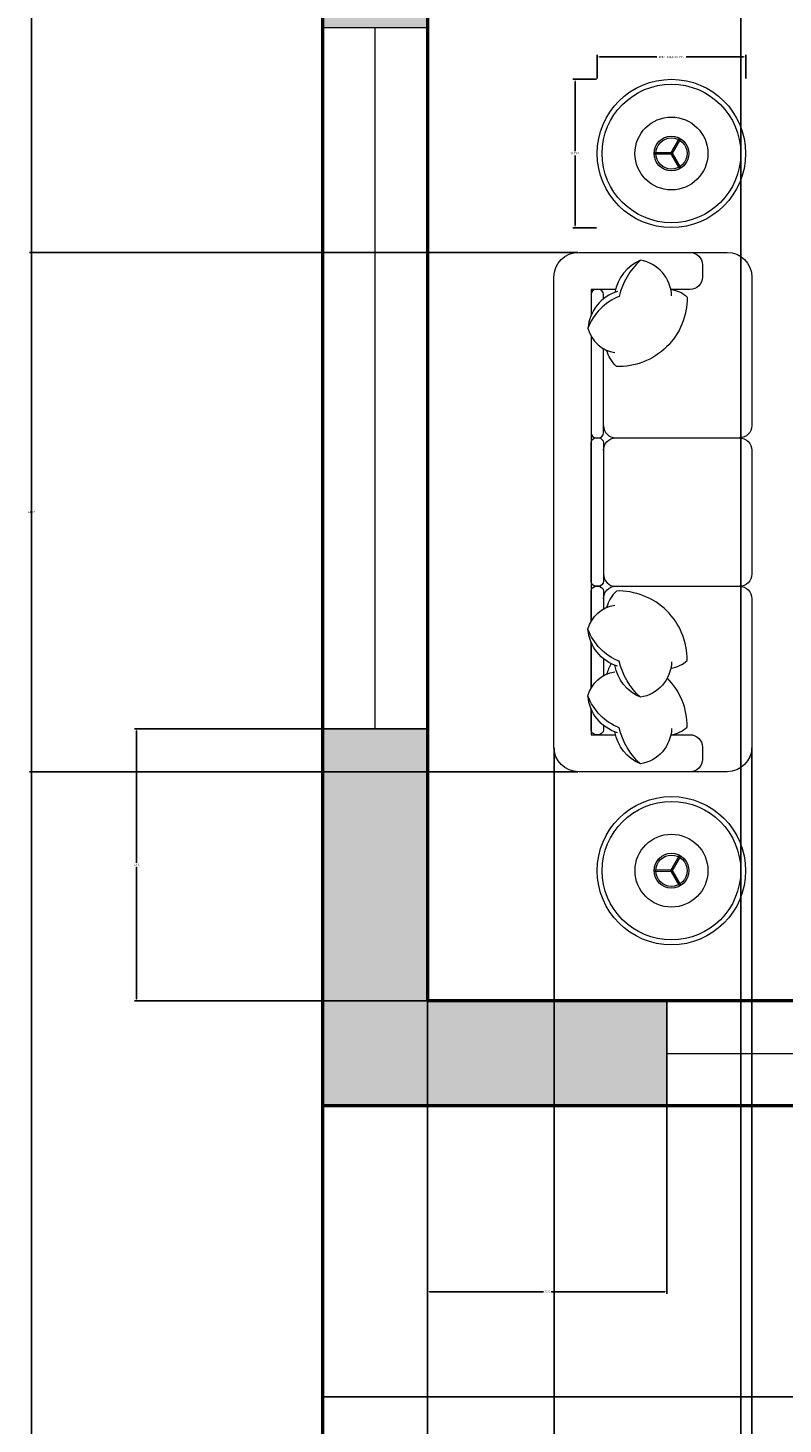
# Model space of a CAD drawing. Units: inches. Extents: x 3 to 380, y -485 to 60.
# Tile 2 of 8: x 3 to 67, y -390 to -270. Entities that reach past the tile are written whole.
import ezdxf

# ---------------------------------------------------------------- set-up
doc = ezdxf.new("R2010")
doc.units = ezdxf.units.IN
doc.header["$MEASUREMENT"] = 0
for name, color, linetype, lineweight in [('A-ANNO-DIMS', 2, 'Continuous', 18), ('A-FURN', 8, 'Continuous', 18), ('A-GLAZ', 4, 'Continuous', 18), ('A-WALL', 7, 'Continuous', 50), ('A-WALL-PATT', 252, 'Continuous', 13)]:
    doc.layers.add(name, color=color, linetype=linetype, lineweight=lineweight)
doc.styles.get("Standard").update_dxf_attribs({"font": 'arial.ttf'})
doc.dimstyles.get("Standard").update_dxf_attribs({"dimtxt": 0.18, "dimasz": 0.18, "dimexe": 0.18, "dimexo": 0.0625, "dimgap": 0.09, "dimtad": 0, "dimtih": 1, "dimtoh": 1, "dimdec": 0, "dimzin": 0, "dimdsep": 46, "dimlunit": 3, "dimtxsty": 'Standard', "dimcen": 0.09, "dimadec": 0, "dimazin": 0, "dimtfac": 1, "dimtdec": 0, "dimtofl": 0, "dimtmove": 0, "dimatfit": 3, "dimfxl": 1, "dimtolj": 1, "dimtzin": 0, "dimarcsym": 0})

# ---------------------------------------------------------------- blocks, each defined once
blk = doc.blocks.new('LIVING-END-TABLE')
at = {"ltscale": 0.03}
for p, q in [((6.3, 6.39), (7.04, 7.68)), ((6.41, 6.32), (7.16, 7.61)), ((6.35, 6.42), (4.86, 6.42)), ((6.35, 6.29), (4.86, 6.29)), ((6.3, 6.32), (7.04, 5.03)), ((6.41, 6.39), (7.16, 5.09))]:
    blk.add_line(p, q, dxfattribs=at)
for radius in [6.35, 3.12, 1.49, 1.34]:
    blk.add_circle((6.35, 6.35), radius, dxfattribs=at)
blk.add_circle((6.35, 6.35), 5.93)
blk = doc.blocks.new('WIN-60X9')
for p, q in [((60, 9), (0, 9)), ((0, 9), (0, 0)), ((60, 0), (60, 9)), ((0, 4.5), (60, 4.5)), ((0, 0), (60, 0))]:
    blk.add_line(p, q)
blk = doc.blocks.new('WIN-60X9-SPLIT-JAMB')
for p, q in [((60, 9), (0, 9)), ((0, 9), (0, 0)), ((60, 4.5), (60, 9)), ((0, 4.5), (60, 4.5)), ((60, 4.5), (60, 0)), ((0, 0), (60, 0))]:
    blk.add_line(p, q)
blk = doc.blocks.new('*D37')
at = {"layer": 'A-ANNO-DIMS', "color": 0, "lineweight": -2, "transparency": 16777216}
for p, q in [((51.37, -274.46), (51.37, -272.43)), ((64.08, -274.46), (64.08, -272.43)), ((51.55, -272.61), (56.47, -272.61)), ((63.9, -272.61), (58.98, -272.61))]:
    blk.add_line(p, q, dxfattribs=at)
at = {"layer": 'A-ANNO-DIMS', "color": 0, "transparency": 16777216}
for points in [[(51.55, -272.58), (51.55, -272.64), (51.37, -272.61)], [(63.9, -272.58), (63.9, -272.64), (64.08, -272.61)]]:
    blk.add_solid(points, dxfattribs=at)
at = {"layer": 'Defpoints', "color": 0, "transparency": 16777216}
for p in [(64.08, -272.61), (51.37, -274.52), (64.08, -274.52)]:
    blk.add_point(p, dxfattribs=at)
at = {"layer": 'A-ANNO-DIMS', "color": 0, "transparency": 16777216, "insert": (57.72, -272.61), "char_height": 0.18, "attachment_point": 5}
blk.add_mtext('\\A1;END TABLE 13 TYP.', dxfattribs=at)
blk = doc.blocks.new('*D38')
at = {"layer": 'A-ANNO-DIMS', "color": 0, "lineweight": -2, "transparency": 16777216}
for p, q in [((51.31, -274.52), (49.29, -274.52)), ((49.47, -274.7), (49.47, -280.69)), ((49.47, -287.05), (49.47, -281.06)), ((51.31, -287.23), (49.29, -287.23))]:
    blk.add_line(p, q, dxfattribs=at)
at = {"layer": 'A-ANNO-DIMS', "color": 0, "transparency": 16777216}
for points in [[(49.44, -274.7), (49.5, -274.7), (49.47, -274.52)], [(49.44, -287.05), (49.5, -287.05), (49.47, -287.23)]]:
    blk.add_solid(points, dxfattribs=at)
at = {"layer": 'Defpoints', "color": 0, "transparency": 16777216}
for p in [(49.47, -274.52), (51.37, -274.52), (51.37, -287.23)]:
    blk.add_point(p, dxfattribs=at)
at = {"layer": 'A-ANNO-DIMS', "color": 0, "transparency": 16777216, "insert": (49.47, -280.87), "char_height": 0.18, "attachment_point": 5}
blk.add_mtext('\\A1;13 TYP.', dxfattribs=at)
blk = doc.blocks.new('*D50')
at = {"layer": 'A-ANNO-DIMS', "color": 0, "lineweight": -2, "transparency": 16777216}
for p, q in [((27.78, 15.16), (2.76, 15.16)), ((2.94, 14.98), (2.94, -222.4)), ((2.94, -460.16), (2.94, -222.77)), ((27.78, -460.34), (2.76, -460.34))]:
    blk.add_line(p, q, dxfattribs=at)
at = {"layer": 'A-ANNO-DIMS', "color": 0, "transparency": 16777216}
for points in [[(2.91, 14.98), (2.97, 14.98), (2.94, 15.16)], [(2.91, -460.16), (2.97, -460.16), (2.94, -460.34)]]:
    blk.add_solid(points, dxfattribs=at)
at = {"layer": 'Defpoints', "color": 0, "transparency": 16777216}
for p in [(2.94, 15.16), (27.84, 15.16), (27.84, -460.34)]:
    blk.add_point(p, dxfattribs=at)
at = {"layer": 'A-ANNO-DIMS', "color": 0, "transparency": 16777216, "insert": (2.94, -222.59), "char_height": 0.18, "attachment_point": 5}
blk.add_mtext('\\A1;475.5', dxfattribs=at)
blk = doc.blocks.new('*D52')
at = {"layer": 'A-ANNO-DIMS', "color": 0, "lineweight": -2, "transparency": 16777216}
for p, q in [((27.84, -362.49), (27.84, -387.51)), ((168.84, -362.49), (168.84, -387.51)), ((28.02, -387.33), (98.08, -387.33)), ((168.66, -387.33), (98.6, -387.33))]:
    blk.add_line(p, q, dxfattribs=at)
at = {"layer": 'A-ANNO-DIMS', "color": 0, "transparency": 16777216}
for points in [[(28.02, -387.3), (28.02, -387.36), (27.84, -387.33)], [(168.66, -387.3), (168.66, -387.36), (168.84, -387.33)]]:
    blk.add_solid(points, dxfattribs=at)
at = {"layer": 'Defpoints', "color": 0, "transparency": 16777216}
for p in [(27.84, -362.43), (168.84, -362.43), (27.84, -387.33)]:
    blk.add_point(p, dxfattribs=at)
at = {"layer": 'A-ANNO-DIMS', "color": 0, "transparency": 16777216, "insert": (98.34, -387.33), "char_height": 0.18, "attachment_point": 5}
blk.add_mtext('\\A1;141', dxfattribs=at)
blk = doc.blocks.new('*D55')
at = {"layer": 'A-ANNO-DIMS', "color": 0, "lineweight": -2, "transparency": 16777216}
for p, q in [((36.78, -330.13), (11.76, -330.13)), ((11.94, -330.31), (11.94, -341.6)), ((11.94, -353.25), (11.94, -341.96)), ((36.78, -353.43), (11.76, -353.43))]:
    blk.add_line(p, q, dxfattribs=at)
at = {"layer": 'A-ANNO-DIMS', "color": 0, "transparency": 16777216}
for points in [[(11.91, -330.31), (11.97, -330.31), (11.94, -330.13)], [(11.91, -353.25), (11.97, -353.25), (11.94, -353.43)]]:
    blk.add_solid(points, dxfattribs=at)
at = {"layer": 'Defpoints', "color": 0, "transparency": 16777216}
for p in [(11.94, -330.13), (36.84, -330.13), (36.84, -353.43)]:
    blk.add_point(p, dxfattribs=at)
at = {"layer": 'A-ANNO-DIMS', "color": 0, "transparency": 16777216, "insert": (11.94, -341.78), "char_height": 0.18, "attachment_point": 5}
blk.add_mtext('\\A1;23.3', dxfattribs=at)
blk = doc.blocks.new('*D81')
at = {"layer": 'A-ANNO-DIMS', "color": 0, "lineweight": -2, "transparency": 16777216}
for p, q in [((36.84, -353.49), (36.84, -378.51)), ((57.34, -353.49), (57.34, -378.51)), ((37.02, -378.33), (46.76, -378.33)), ((57.16, -378.33), (47.42, -378.33))]:
    blk.add_line(p, q, dxfattribs=at)
at = {"layer": 'A-ANNO-DIMS', "color": 0, "transparency": 16777216}
for points in [[(37.02, -378.3), (37.02, -378.36), (36.84, -378.33)], [(57.16, -378.3), (57.16, -378.36), (57.34, -378.33)]]:
    blk.add_solid(points, dxfattribs=at)
at = {"layer": 'Defpoints', "color": 0, "transparency": 16777216}
for p in [(36.84, -353.43), (57.34, -353.43), (36.84, -378.33)]:
    blk.add_point(p, dxfattribs=at)
at = {"layer": 'A-ANNO-DIMS', "color": 0, "transparency": 16777216, "insert": (47.09, -378.33), "char_height": 0.18, "attachment_point": 5}
blk.add_mtext('\\A1;20.5', dxfattribs=at)
blk = doc.blocks.new('*D92')
at = {"layer": 'A-ANNO-DIMS', "color": 0, "lineweight": -2, "transparency": 16777216}
for p, q in [((36.84, -85.2), (36.84, -485.42)), ((63.65, -85.2), (63.65, -485.42)), ((37.02, -485.24), (49.87, -485.24)), ((63.47, -485.24), (50.62, -485.24))]:
    blk.add_line(p, q, dxfattribs=at)
at = {"layer": 'A-ANNO-DIMS', "color": 0, "transparency": 16777216}
for points in [[(37.02, -485.21), (37.02, -485.27), (36.84, -485.24)], [(63.47, -485.21), (63.47, -485.27), (63.65, -485.24)]]:
    blk.add_solid(points, dxfattribs=at)
at = {"layer": 'Defpoints', "color": 0, "transparency": 16777216}
for p in [(36.84, -85.14), (63.65, -85.14), (63.65, -485.24)]:
    blk.add_point(p, dxfattribs=at)
at = {"layer": 'A-ANNO-DIMS', "color": 0, "transparency": 16777216, "insert": (50.24, -485.24), "char_height": 0.18, "attachment_point": 5}
blk.add_mtext('\\A1;26.81', dxfattribs=at)
blk = doc.blocks.new('*D97')
at = {"layer": 'A-ANNO-DIMS', "color": 0, "lineweight": -2, "transparency": 16777216}
for p, q in [((49.72069, -289.344461), (2.760351, -289.344461)), ((2.940351, -289.524461), (2.940351, -311.400545)), ((2.940351, -333.636629), (2.940351, -311.760545)), ((49.72069, -333.816629), (2.760351, -333.816629))]:
    blk.add_line(p, q, dxfattribs=at)
at = {"layer": 'A-ANNO-DIMS', "color": 0, "transparency": 16777216}
for points in [[(2.910351, -289.524461), (2.970351, -289.524461), (2.940351, -289.344461)], [(2.910351, -333.636629), (2.970351, -333.636629), (2.940351, -333.816629)]]:
    blk.add_solid(points, dxfattribs=at)
at = {"layer": 'Defpoints', "color": 0, "transparency": 16777216}
for p in [(49.78319, -289.344461), (2.940351, -333.816629), (49.78319, -333.816629)]:
    blk.add_point(p, dxfattribs=at)
at = {"layer": 'A-ANNO-DIMS', "color": 0, "transparency": 16777216, "insert": (2.940351, -311.580545), "char_height": 0.18, "attachment_point": 5}
blk.add_mtext('\\A1;44.47', dxfattribs=at)
blk = doc.blocks.new('*D98')
at = {"layer": 'A-ANNO-DIMS', "color": 0, "lineweight": -2, "transparency": 16777216}
for p, q in [((47.67, -331.76), (47.67, -485.42)), ((64.61, -331.76), (64.61, -485.42)), ((47.85, -485.24), (55.68, -485.24)), ((64.43, -485.24), (56.59, -485.24))]:
    blk.add_line(p, q, dxfattribs=at)
at = {"layer": 'A-ANNO-DIMS', "color": 0, "transparency": 16777216}
for points in [[(47.85, -485.21), (47.85, -485.27), (47.67, -485.24)], [(64.43, -485.21), (64.43, -485.27), (64.61, -485.24)]]:
    blk.add_solid(points, dxfattribs=at)
at = {"layer": 'Defpoints', "color": 0, "transparency": 16777216}
for p in [(47.67, -331.7), (64.61, -331.7), (64.61, -485.24)]:
    blk.add_point(p, dxfattribs=at)
at = {"layer": 'A-ANNO-DIMS', "color": 0, "transparency": 16777216, "insert": (56.14, -485.24), "char_height": 0.18, "attachment_point": 5}
blk.add_mtext('\\A1;16.942', dxfattribs=at)

msp = doc.modelspace()

# ---------------------------------------------------------------- hatches: boundary and pattern name
at = {"layer": 'A-WALL-PATT'}
h = msp.add_hatch(color=256, dxfattribs=at)
h.dxf.hatch_style = 1
h.paths.add_polyline_path([(36.8404, 6.1643), (51.3404, 6.1643), (51.3404, 15.1643), (27.8404, 15.1643), (27.8404, -143.6318), (36.8404, -143.6318)])
h.paths.add_polyline_path([(125.8404, 10.6643), (125.8404, 15.1643), (111.3404, 15.1643), (111.3404, 6.1643), (125.8404, 6.1643)])
h.paths.add_polyline_path([(170.6358, 15.1643), (153.8404, 15.1643), (153.8404, 6.1643), (156.8404, 6.1643), (156.8404, -82.3357), (173.3404, -82.3357), (173.3404, -130.3357), (177.8404, -130.3357), (180.8404, -130.3357), (180.8404, -125.8357), (177.8404, -125.8357), (177.8404, -82.3357), (201.8404, -82.3357), (201.8404, -38.0857), (197.3404, -38.0857), (197.3404, -77.8357), (161.3404, -77.8357), (161.3404, 6.1643), (170.6358, 6.1643)])
h.paths.add_polyline_path([(241.3739, 15.1643), (194.6358, 15.1643), (194.6358, 6.1643), (241.3739, 6.1643)])
h.paths.add_polyline_path([(201.8404, 6.1643), (197.3404, 6.1643), (197.3404, -12.1977), (201.8404, -12.1977)], flags=17)
h.paths.add_polyline_path([(354.8404, 15.1643), (301.3739, 15.1643), (301.3739, 6.1643), (345.8404, 6.1643), (345.8404, -34.0336), (354.8404, -34.0336)])
h.paths.add_polyline_path([(354.8404, -94.0336), (345.8404, -94.0336), (345.8404, -159.3738), (354.8404, -159.3738)])
h.paths.add_polyline_path([(345.8404, -125.8357), (209.3404, -125.8357), (209.3404, -205.8357), (211.5904, -205.8357), (213.8404, -205.8357), (213.8404, -130.3357), (345.8404, -130.3357)])
h.paths.add_polyline_path([(36.8404, -203.6318), (27.8404, -203.6318), (27.8404, -270.1269), (36.8404, -270.1269)])
h.paths.add_polyline_path([(36.8404, -330.1269), (27.8404, -330.1269), (27.8404, -362.428), (57.3404, -362.428), (57.3404, -353.428), (36.8404, -353.428)])
h.paths.add_polyline_path([(177.8404, -331.3357), (180.8404, -331.3357), (180.8404, -326.8357), (173.3404, -326.8357), (173.3404, -353.428), (165.8404, -353.428), (165.8404, -362.428), (168.8404, -362.428), (168.8404, -451.3357), (168.8404, -460.3357), (231.8404, -460.3357), (231.8404, -451.3357), (177.8404, -451.3357)])
h.paths.add_polyline_path([(354.8404, -305.1003), (345.8404, -305.1003), (345.8404, -363.2829), (354.8404, -363.2829)])
h.paths.add_polyline_path([(345.8404, -326.8357), (213.8404, -326.8357), (213.8404, -312.8357), (211.5904, -312.8357), (209.3404, -312.8357), (209.3404, -331.3357), (345.8404, -331.3357)])
h.paths.add_polyline_path([(345.8404, -262.3357), (237.8404, -262.3357), (237.8404, -233.8357), (209.3404, -233.8357), (209.3404, -284.8357), (213.8404, -284.8357), (213.8404, -238.3357), (233.3404, -238.3357), (233.3404, -266.8357), (345.8404, -266.8357)])
h.paths.add_polyline_path([(354.8404, -219.3738), (345.8404, -219.3738), (345.8404, -281.1003), (354.8404, -281.1003)])

# ---------------------------------------------------------------- linework, layer by layer
at = {"layer": 'A-FURN', "ltscale": 0.03}
msp.add_lwpolyline([(62.4895, -289.3445, -0.41421356), (64.6072, -291.4622), (64.6072, -304.1685, -0.41421356), (63.5484, -305.2274, -0.41421356), (64.6072, -306.2862), (64.6072, -316.8749, -0.41421356), (63.5484, -317.9337, -0.41421356), (64.6072, -318.9926), (64.6072, -331.6989, -0.41421356), (62.4895, -333.8166), (49.7832, -333.8166, -0.41421356), (47.6655, -331.6989), (47.6655, -291.4622, -0.41421356), (49.7832, -289.3445)], format="xyb", close=True, dxfattribs=at)
at = {"layer": 'A-FURN'}
for points in [[(55.0675, -290.0184, 0.14772988), (53.2477, -293.1131, 0.21334276), (50.5787, -295.8438, 0.17866181)], [(57.7365, -293.0524, 0.35677236), (55.0675, -290.0184, 0.24954205), (52.868, -292.7675, -9.61688035)], [(59.3129, -289.3445, -0.41421356), (60.3718, -290.4033), (60.3718, -291.4622, -0.41421356), (59.3129, -292.521), (57.6724, -292.521)], [(53.1027, -292.6856, 0.30666349), (50.5787, -295.8438, 0.30632997), (52.8838, -297.9069, -0.87284716)], [(51.9009, -293.3291), (51.9009, -292.9446, 0.41421356), (51.4774, -292.521), (51.2656, -292.521, 0.41421356), (50.8421, -292.9446)], [(57.6719, -292.5187, -0.16554063), (59.071, -293.1738, -0.42598917), (53.0051, -299.1206, -0.12152332), (52.169, -297.7089, 7.11546429)], [(50.8421, -292.9446), (50.8421, -294.7486, 0.41421356)], [(50.8421, -296.5102), (50.8421, -304.8038, 0.41421356), (51.2656, -305.2274), (51.4774, -305.2274, 0.41421356), (51.9009, -304.8038), (51.9009, -297.5764, 0.41421356)], [(51.9009, -304.1685, 0.41421356), (52.9598, -305.2274), (63.5484, -305.2274, 0.41421356)], [(51.9009, -306.2862, -0.41421356), (52.9598, -305.2274)], [(50.8421, -320.9469), (50.8421, -318.3573, -0.41421356), (51.2656, -317.9337), (51.4774, -317.9337, -0.41421356), (51.9009, -318.3573), (51.9009, -319.8807, -0.41421356)], [(51.9009, -316.8749, 0.41421356), (52.9598, -317.9337)], [(51.9009, -318.9926, -0.41421356), (52.9598, -317.9337), (63.5484, -317.9337, -0.41421356)], [(57.6719, -324.9383, 0.16554063), (59.071, -324.2833, 0.42598917), (53.0051, -318.3365, 0.12152332), (52.169, -319.7481, -7.11546429)], [(53.1027, -324.7715, -0.30666349), (50.5787, -321.6133, -0.30632997), (52.8838, -319.5501, 0.87284716)], [(55.0675, -327.4387, -0.14772988), (53.2477, -324.3439, -0.21334276), (50.5787, -321.6133, -0.17866181)], [(50.8421, -326.6509), (50.8421, -322.7085, -0.41421356)], [(51.9009, -324.128), (51.9009, -325.5847, -0.41421356)], [(52.583, -324.5644, 0.07186538), (52.169, -325.4522, -7.11546429)], [(57.7365, -324.4046, -0.35677236), (55.0675, -327.4387, -0.24954205), (52.868, -324.6895, 9.61688035)], [(53.1027, -330.4755, -0.30666349), (50.5787, -327.3173, -0.30632997), (52.8838, -325.2542, 0.87284716)], [(57.6719, -330.6423, 0.16554063), (59.071, -329.9873, 0.20023115), (57.367, -325.784, 0.12152332)], [(55.0675, -333.1427, -0.14772988), (53.2477, -330.048, -0.21334276), (50.5787, -327.3173, -0.17866181)], [(50.8421, -328.4125), (50.8421, -330.64), (52.923, -330.64, -0.41421356)], [(50.8421, -330.2165), (50.8421, -328.4125, -0.41421356)], [(51.9009, -329.832), (51.9009, -330.2165, -0.41421356), (51.4774, -330.64), (51.2656, -330.64, -0.41421356), (50.8421, -330.2165)], [(57.7365, -330.1087, -0.35677236), (55.0675, -333.1427, -0.24954205), (52.868, -330.3936, 9.61688035)], [(57.6724, -330.64), (59.3129, -330.64, -0.41421356), (60.3718, -331.6989), (60.3718, -332.7578, -0.41421356), (59.3129, -333.8166)]]:
    msp.add_lwpolyline(points, format="xyb", dxfattribs=at)
for points in [[(52.923, -292.521), (50.8421, -292.521), (50.8421, -294.7486)], [(50.8421, -296.5102), (50.8421, -320.9469)], [(50.8421, -322.7085), (50.8421, -326.6509)]]:
    msp.add_lwpolyline(points, dxfattribs=at)
msp.add_lwpolyline([(50.8421, -317.5102), (50.8421, -305.6509, -0.41421356), (51.2656, -305.2274), (51.4774, -305.2274, -0.41421356), (51.9009, -305.6509), (51.9009, -317.5102, -0.41421356), (51.4774, -317.9337), (51.2656, -317.9337, -0.41421356)], format="xyb", close=True, dxfattribs=at)
at = {"layer": 'A-WALL'}
for p, q in [((27.8404, 15.1643), (27.8404, -460.3357)), ((36.8404, 6.1643), (36.8404, -353.428)), ((137.8404, -353.428), (36.8404, -353.428)), ((137.8404, -362.428), (27.8404, -362.428))]:
    msp.add_line(p, q, dxfattribs=at)

# ---------------------------------------------------------------- block references
at = {"layer": 'A-FURN'}
msp.add_blockref('LIVING-END-TABLE', (51.371, -287.227), dxfattribs=at)
at = {"layer": 'A-FURN', "rotation": 239.9999999970145}
msp.add_blockref('LIVING-END-TABLE', (55.3992, -333.6084), dxfattribs=at)
at = {"layer": 'A-GLAZ', "rotation": 270}
msp.add_blockref('WIN-60X9', (27.84, -270.127), dxfattribs=at)
at = {"layer": 'A-GLAZ'}
msp.add_blockref('WIN-60X9-SPLIT-JAMB', (57.34, -362.4283), dxfattribs=at)

# ---------------------------------------------------------------- dimensions: what is measured, and where the dimension line sits
at = {"layer": 'A-ANNO-DIMS'}
for base, p1, p2, angle, override, picture, middle in [((2.9404, 15.1643), (27.8404, -460.3357), (27.8404, 15.1643), 90, {"dimdec": 1, "dimlfac": 1, "dimrnd": 0, "dimzin": 0, "dimdsep": 46, "dimlunit": 2}, '*D50', (2.9404, -222.5857)), ((2.9404, -333.8166), (49.7832, -289.3445), (49.7832, -333.8166), 90, {"dimdec": 2, "dimlfac": 1, "dimrnd": 0, "dimzin": 0, "dimdsep": 46, "dimlunit": 2}, '*D97', (2.9404, -311.5805)), ((11.9404, -330.1269), (36.8404, -353.428), (36.8404, -330.1269), 90, {"dimdec": 1, "dimlfac": 1, "dimrnd": 0, "dimzin": 0, "dimdsep": 46, "dimlunit": 2}, '*D55', (11.9404, -341.7774)), ((36.8404, -378.328), (57.3404, -353.428), (36.8404, -353.428), 180, {"dimdec": 1, "dimlfac": 1, "dimrnd": 0, "dimzin": 0, "dimdsep": 46, "dimlunit": 2}, '*D81', (47.0904, -378.328)), ((27.8404, -387.328), (168.8404, -362.428), (27.8404, -362.428), 180, {"dimdec": 0, "dimlfac": 1, "dimrnd": 0, "dimzin": 0, "dimdsep": 46, "dimlunit": 2}, '*D52', (98.3404, -387.328))]:
    dim = msp.add_linear_dim(base=base, p1=p1, p2=p2, angle=angle, dimstyle='Standard', override=override, dxfattribs=at)
    dim.commit()
    dim.dimension.update_dxf_attribs({"geometry": picture, "text_midpoint": middle})
for base, p1, p2, override, picture, middle in [((63.6489, -485.2357), (36.8404, -85.1388), (63.6489, -85.1388), {"dimdec": 2, "dimlfac": 1, "dimrnd": 0, "dimzin": 0, "dimdsep": 46, "dimlunit": 2}, '*D92', (50.2446, -485.2357)), ((64.6072, -485.2357), (47.6655, -331.6989), (64.6072, -331.6989), {"dimdec": 3, "dimlfac": 1, "dimrnd": 0, "dimzin": 0, "dimdsep": 46, "dimlunit": 2}, '*D98', (56.1364, -485.2357))]:
    dim = msp.add_linear_dim(base=base, p1=p1, p2=p2, dimstyle='Standard', override=override, dxfattribs=at)
    dim.commit()
    dim.dimension.update_dxf_attribs({"geometry": picture, "text_midpoint": middle})
dim = msp.add_linear_dim(base=(64.0778, -272.6145), p1=(51.3715, -274.5204), p2=(64.0778, -274.5204), text='END TABLE <> TYP.', dimstyle='Standard', override={"dimdec": 0, "dimlfac": 1, "dimrnd": 0, "dimzin": 0, "dimdsep": 46, "dimlunit": 2}, dxfattribs=at)
dim.commit()
dim.dimension.update_dxf_attribs({"geometry": '*D37', "text_midpoint": (57.7246, -272.6145)})
dim = msp.add_linear_dim(base=(49.4655, -274.5204), p1=(51.3715, -287.2267), p2=(51.3715, -274.5204), angle=90, text='<> TYP.', dimstyle='Standard', override={"dimdec": 0, "dimlfac": 1, "dimrnd": 0, "dimzin": 0, "dimdsep": 46, "dimlunit": 2}, dxfattribs=at)
dim.commit()
dim.dimension.update_dxf_attribs({"geometry": '*D38', "text_midpoint": (49.4655, -280.8736)})

doc.saveas('drawing.dxf')
